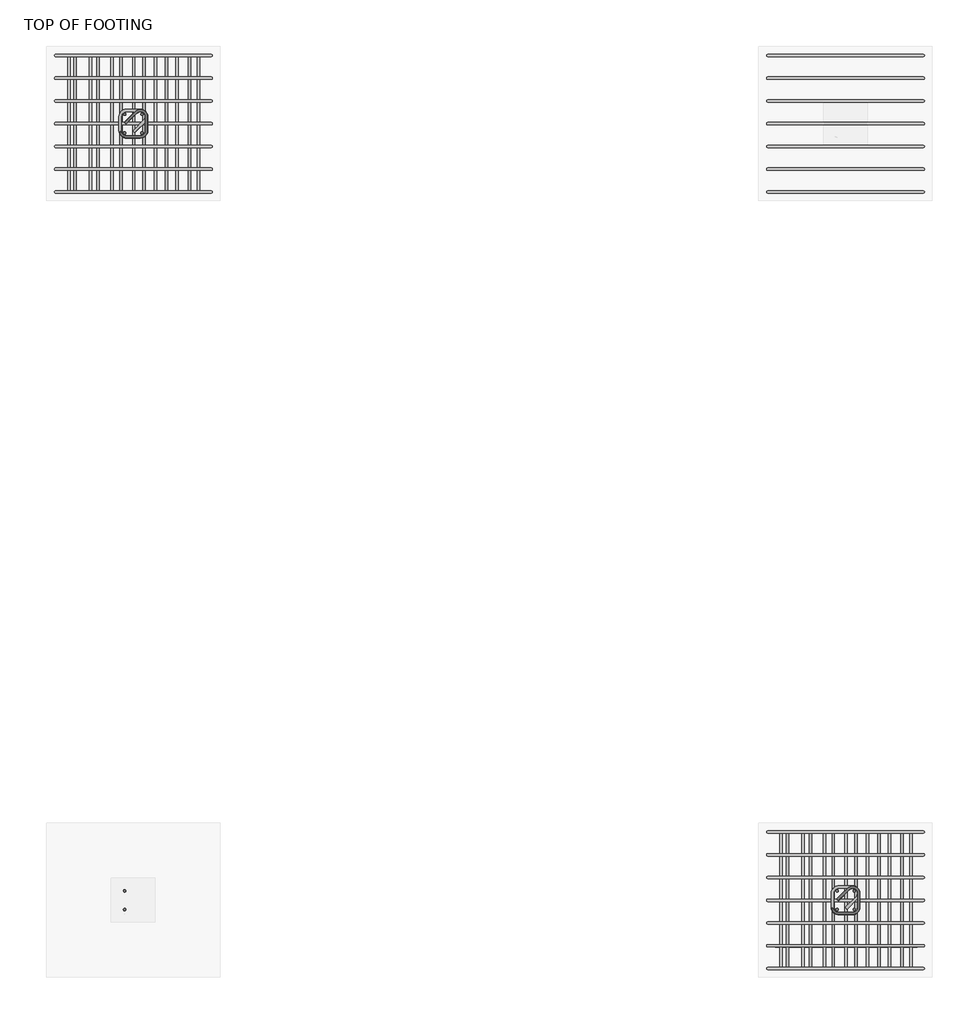
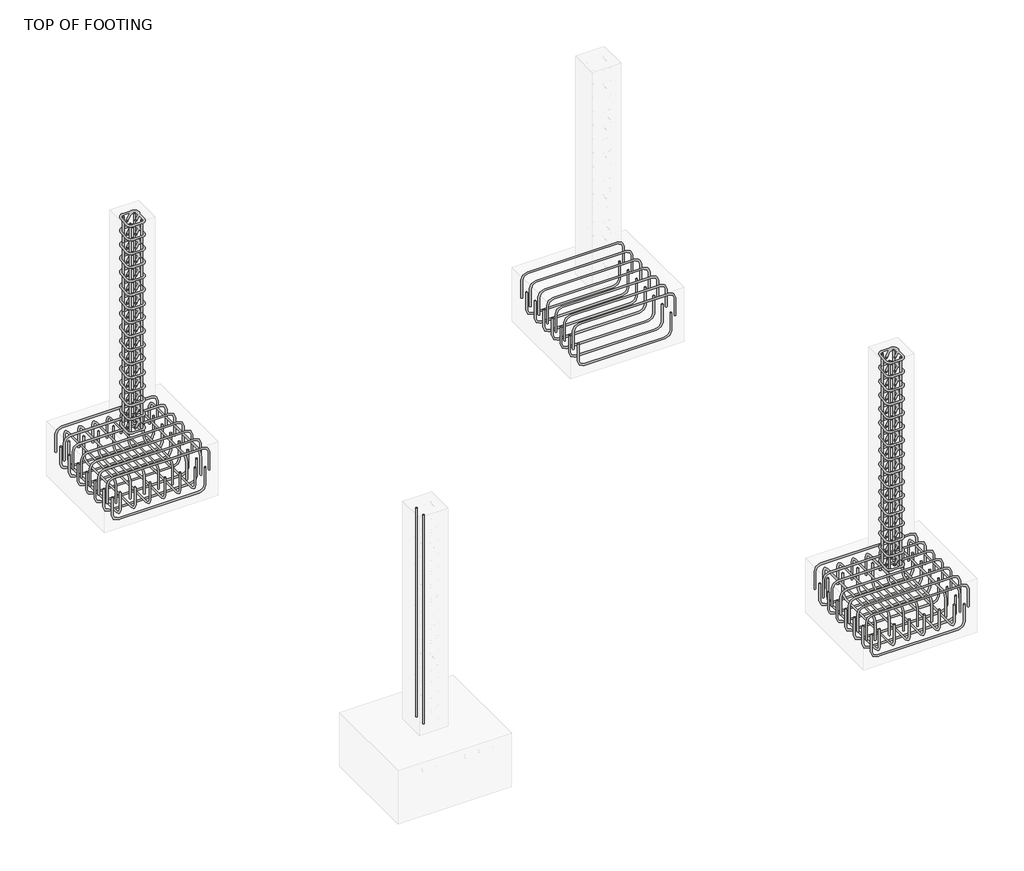
# One storey, part 4 of 6: 17 reinforcing bars.
"""IFC4 building model written with IfcOpenShell, lengths in millimetres."""

from ifc_helpers import new_model, si_unit, point, frame, origin, place, context, project, spatial, polyline, circle_curve, trimmed, segment, composite_curve, source, transform, mapped, element, save
from ifc_brep_helpers import swept_disk

model = new_model("IFC4")

# Units and contexts
model_context = context("Model", 3, world=origin())
ifc_project = project(units=[si_unit("LENGTHUNIT", "METRE", prefix="MILLI")], contexts=[model_context])

# Site, building, storey
site = spatial("IfcSite", under=ifc_project)
building = spatial("IfcBuilding", under=site)
storey = spatial("IfcBuildingStorey", under=building, Name="TOP OF FOOTING", Elevation=-1828.8)

# Reinforcing bars
placement = place(None, origin())
reinforcing_bar_shape = source(origin(), model_context, "Body", "SolidModel", [
    swept_disk(composite_curve([segment(polyline([(-6942.8971795, 120.9474721, -2038.8), (-6942.8971795, 120.9474721, -2186.1)]), True, "CONTINUOUS"), segment(trimmed(circle_curve(frame((-6989.2471795, 120.9474721, -2186.1), z_axis=(0.0, 1.0, 0.0), x_axis=(46.350000000000364, 0.0, 0.0)), 46.35), [point((-6942.8971795, 120.9474721, -2186.1))], [point((-6989.2471795, 120.9474721, -2232.45))], True, "CARTESIAN"), True, "CONTINUOUS"), segment(polyline([(-6989.2471795, 120.9474721, -2232.45), (-7632.3877906, 120.9474721, -2232.45)]), True, "CONTINUOUS"), segment(trimmed(circle_curve(frame((-7632.3877906, 120.9474721, -2186.1), z_axis=(0.0, 1.0, 0.0), x_axis=(0.0, 0.0, -46.34999999999991)), 46.35), [point((-7632.3877906, 120.9474721, -2232.45))], [point((-7678.7377906, 120.9474721, -2186.1))], True, "CARTESIAN"), True, "CONTINUOUS"), segment(polyline([(-7678.7377906, 120.9474721, -2186.1), (-7678.7377906, 120.9474721, -2038.8)]), True, "CONTINUOUS")], self_intersect=False), 6.35),
])
element("IfcReinforcingBar", 1, at=placement, inside=storey, context=model_context, shape_type="MappedRepresentation", body=[
    mapped(reinforcing_bar_shape, transform((0.0, 0.0, 0.0), x_axis=(1.0, 0.0, 0.0), y_axis=(0.0, 1.0, 0.0), z_axis=(0.0, 0.0, 1.0))),
    mapped(reinforcing_bar_shape, transform((0.0, -117.8833333, 0.0), x_axis=(1.0, 0.0, 0.0), y_axis=(0.0, 1.0, 0.0), z_axis=(0.0, 0.0, 1.0))),
    mapped(reinforcing_bar_shape, transform((0.0, -235.7666667, 0.0), x_axis=(1.0, 0.0, 0.0), y_axis=(0.0, 1.0, 0.0), z_axis=(0.0, 0.0, 1.0))),
    mapped(reinforcing_bar_shape, transform((0.0, -353.65, 0.0), x_axis=(1.0, 0.0, 0.0), y_axis=(0.0, 1.0, 0.0), z_axis=(0.0, 0.0, 1.0))),
    mapped(reinforcing_bar_shape, transform((0.0, -471.5333333, 0.0), x_axis=(1.0, 0.0, 0.0), y_axis=(0.0, 1.0, 0.0), z_axis=(0.0, 0.0, 1.0))),
    mapped(reinforcing_bar_shape, transform((0.0, -589.4166667, 0.0), x_axis=(1.0, 0.0, 0.0), y_axis=(0.0, 1.0, 0.0), z_axis=(0.0, 0.0, 1.0))),
    mapped(reinforcing_bar_shape, transform((0.0, -707.3, 0.0), x_axis=(1.0, 0.0, 0.0), y_axis=(0.0, 1.0, 0.0), z_axis=(0.0, 0.0, 1.0))),
])
reinforcing_bar_2_shape = source(origin(), model_context, "Body", "SolidModel", [
    swept_disk(composite_curve([segment(polyline([(-7718.1173382, 120.9474721, -2070.9463075), (-7718.1173382, 120.9474721, -1923.6463075)]), True, "CONTINUOUS"), segment(trimmed(circle_curve(frame((-7671.7673382, 120.9474721, -1923.6463075), z_axis=(0.0, 1.0, 0.0), x_axis=(-46.349999999999454, 0.0, 0.0)), 46.35), [point((-7718.1173382, 120.9474721, -1923.6463075))], [point((-7671.7673382, 120.9474721, -1877.2963075))], True, "CARTESIAN"), True, "CONTINUOUS"), segment(polyline([(-7671.7673382, 120.9474721, -1877.2963075), (-6957.1673382, 120.9474721, -1877.2963075)]), True, "CONTINUOUS"), segment(trimmed(circle_curve(frame((-6957.1673382, 120.9474721, -1923.6463075), z_axis=(0.0, 1.0, 0.0), x_axis=(0.0, 0.0, 46.34999999999991)), 46.35), [point((-6957.1673382, 120.9474721, -1877.2963075))], [point((-6910.8173382, 120.9474721, -1923.6463075))], True, "CARTESIAN"), True, "CONTINUOUS"), segment(polyline([(-6910.8173382, 120.9474721, -1923.6463075), (-6910.8173382, 120.9474721, -2070.9463075)]), True, "CONTINUOUS")], self_intersect=False), 6.35),
])
element("IfcReinforcingBar", 2, at=placement, inside=storey, context=model_context, shape_type="MappedRepresentation", body=[
    mapped(reinforcing_bar_2_shape, transform((0.0, 0.0, 0.0), x_axis=(1.0, 0.0, 0.0), y_axis=(0.0, 1.0, 0.0), z_axis=(0.0, 0.0, 1.0))),
    mapped(reinforcing_bar_2_shape, transform((0.0, -117.8833333, 0.0), x_axis=(1.0, 0.0, 0.0), y_axis=(0.0, 1.0, 0.0), z_axis=(0.0, 0.0, 1.0))),
    mapped(reinforcing_bar_2_shape, transform((0.0, -235.7666667, 0.0), x_axis=(1.0, 0.0, 0.0), y_axis=(0.0, 1.0, 0.0), z_axis=(0.0, 0.0, 1.0))),
    mapped(reinforcing_bar_2_shape, transform((0.0, -353.65, 0.0), x_axis=(1.0, 0.0, 0.0), y_axis=(0.0, 1.0, 0.0), z_axis=(0.0, 0.0, 1.0))),
    mapped(reinforcing_bar_2_shape, transform((0.0, -471.5333333, 0.0), x_axis=(1.0, 0.0, 0.0), y_axis=(0.0, 1.0, 0.0), z_axis=(0.0, 0.0, 1.0))),
    mapped(reinforcing_bar_2_shape, transform((0.0, -589.4166667, 0.0), x_axis=(1.0, 0.0, 0.0), y_axis=(0.0, 1.0, 0.0), z_axis=(0.0, 0.0, 1.0))),
    mapped(reinforcing_bar_2_shape, transform((0.0, -707.3, 0.0), x_axis=(1.0, 0.0, 0.0), y_axis=(0.0, 1.0, 0.0), z_axis=(0.0, 0.0, 1.0))),
])
reinforcing_bar_3_shape = source(origin(), model_context, "Body", "SolidModel", [
    swept_disk(composite_curve([segment(polyline([(-6975.9662545, 120.9474721, -2094.0228735), (-6975.9662545, 120.9474721, -1946.7228735)]), True, "CONTINUOUS"), segment(trimmed(circle_curve(frame((-6975.9662545, 74.5974721, -1946.7228735), z_axis=(1.0, 0.0, 0.0), x_axis=(0.0, 46.349999999999994, 0.0)), 46.35), [point((-6975.9662545, 120.9474721, -1946.7228735))], [point((-6975.9662545, 74.5974721, -1900.3728735))], True, "CARTESIAN"), True, "CONTINUOUS"), segment(polyline([(-6975.9662545, 74.5974721, -1900.3728735), (-6975.9662545, -540.0025279, -1900.3728735)]), True, "CONTINUOUS"), segment(trimmed(circle_curve(frame((-6975.9662545, -540.0025279, -1946.7228735), z_axis=(1.0, 0.0, 0.0), x_axis=(0.0, 0.0, 46.350000000000136)), 46.35), [point((-6975.9662545, -540.0025279, -1900.3728735))], [point((-6975.9662545, -586.3525279, -1946.7228735))], True, "CARTESIAN"), True, "CONTINUOUS"), segment(polyline([(-6975.9662545, -586.3525279, -1946.7228735), (-6975.9662545, -586.3525279, -2094.0228735)]), True, "CONTINUOUS")], self_intersect=False), 6.35),
])
element("IfcReinforcingBar", 3, at=placement, inside=storey, context=model_context, shape_type="MappedRepresentation", body=[
    mapped(reinforcing_bar_3_shape, transform((0.0, 0.0, 0.0), x_axis=(1.0, 0.0, 0.0), y_axis=(0.0, 1.0, 0.0), z_axis=(0.0, 0.0, 1.0))),
    mapped(reinforcing_bar_3_shape, transform((-112.124631, 0.0, 0.0), x_axis=(1.0, 0.0, 0.0), y_axis=(0.0, 1.0, 0.0), z_axis=(0.0, 0.0, 1.0))),
    mapped(reinforcing_bar_3_shape, transform((-224.2492621, 0.0, 0.0), x_axis=(1.0, 0.0, 0.0), y_axis=(0.0, 1.0, 0.0), z_axis=(0.0, 0.0, 1.0))),
    mapped(reinforcing_bar_3_shape, transform((-336.3738931, 0.0, 0.0), x_axis=(1.0, 0.0, 0.0), y_axis=(0.0, 1.0, 0.0), z_axis=(0.0, 0.0, 1.0))),
    mapped(reinforcing_bar_3_shape, transform((-448.4985241, 0.0, 0.0), x_axis=(1.0, 0.0, 0.0), y_axis=(0.0, 1.0, 0.0), z_axis=(0.0, 0.0, 1.0))),
    mapped(reinforcing_bar_3_shape, transform((-560.6231552, 0.0, 0.0), x_axis=(1.0, 0.0, 0.0), y_axis=(0.0, 1.0, 0.0), z_axis=(0.0, 0.0, 1.0))),
    mapped(reinforcing_bar_3_shape, transform((-672.7477862, 0.0, 0.0), x_axis=(1.0, 0.0, 0.0), y_axis=(0.0, 1.0, 0.0), z_axis=(0.0, 0.0, 1.0))),
])
reinforcing_bar_4_shape = source(origin(), model_context, "Body", "SolidModel", [
    swept_disk(composite_curve([segment(polyline([(-7615.9564967, 120.9474721, -2014.7438142), (-7615.9564967, 120.9474721, -2162.0438142)]), True, "CONTINUOUS"), segment(trimmed(circle_curve(frame((-7615.9564967, 74.5974721, -2162.0438142), z_axis=(-1.0, 0.0, 0.0), x_axis=(0.0, 46.349999999999994, 0.0)), 46.35), [point((-7615.9564967, 120.9474721, -2162.0438142))], [point((-7615.9564967, 74.5974721, -2208.3938142))], True, "CARTESIAN"), True, "CONTINUOUS"), segment(polyline([(-7615.9564967, 74.5974721, -2208.3938142), (-7615.9564967, -540.0025279, -2208.3938142)]), True, "CONTINUOUS"), segment(trimmed(circle_curve(frame((-7615.9564967, -540.0025279, -2162.0438142), z_axis=(-1.0, 0.0, 0.0), x_axis=(0.0, 0.0, -46.350000000000364)), 46.35), [point((-7615.9564967, -540.0025279, -2208.3938142))], [point((-7615.9564967, -586.3525279, -2162.0438142))], True, "CARTESIAN"), True, "CONTINUOUS"), segment(polyline([(-7615.9564967, -586.3525279, -2162.0438142), (-7615.9564967, -586.3525279, -2014.7438142)]), True, "CONTINUOUS")], self_intersect=False), 6.35),
])
element("IfcReinforcingBar", 4, at=placement, inside=storey, context=model_context, shape_type="MappedRepresentation", body=[
    mapped(reinforcing_bar_4_shape, transform((0.0, 0.0, 0.0), x_axis=(1.0, 0.0, 0.0), y_axis=(0.0, 1.0, 0.0), z_axis=(0.0, 0.0, 1.0))),
    mapped(reinforcing_bar_4_shape, transform((118.647936, 0.0, 0.0), x_axis=(1.0, 0.0, 0.0), y_axis=(0.0, 1.0, 0.0), z_axis=(0.0, 0.0, 1.0))),
    mapped(reinforcing_bar_4_shape, transform((237.295872, 0.0, 0.0), x_axis=(1.0, 0.0, 0.0), y_axis=(0.0, 1.0, 0.0), z_axis=(0.0, 0.0, 1.0))),
    mapped(reinforcing_bar_4_shape, transform((355.943808, 0.0, 0.0), x_axis=(1.0, 0.0, 0.0), y_axis=(0.0, 1.0, 0.0), z_axis=(0.0, 0.0, 1.0))),
    mapped(reinforcing_bar_4_shape, transform((474.591744, 0.0, 0.0), x_axis=(1.0, 0.0, 0.0), y_axis=(0.0, 1.0, 0.0), z_axis=(0.0, 0.0, 1.0))),
    mapped(reinforcing_bar_4_shape, transform((593.23968, 0.0, 0.0), x_axis=(1.0, 0.0, 0.0), y_axis=(0.0, 1.0, 0.0), z_axis=(0.0, 0.0, 1.0))),
])
reinforcing_bar_5_shape = source(origin(), model_context, "Body", "SolidModel", [
    swept_disk(composite_curve([segment(polyline([(-3249.1855212, -3906.2483349, -2038.8), (-3249.1855212, -3906.2483349, -2186.1)]), True, "CONTINUOUS"), segment(trimmed(circle_curve(frame((-3295.5355212, -3906.2483349, -2186.1), z_axis=(0.0, 1.0, 0.0), x_axis=(46.34999999999991, 0.0, 0.0)), 46.35), [point((-3249.1855212, -3906.2483349, -2186.1))], [point((-3295.5355212, -3906.2483349, -2232.45))], True, "CARTESIAN"), True, "CONTINUOUS"), segment(polyline([(-3295.5355212, -3906.2483349, -2232.45), (-3938.6761323, -3906.2483349, -2232.45)]), True, "CONTINUOUS"), segment(trimmed(circle_curve(frame((-3938.6761323, -3906.2483349, -2186.1), z_axis=(0.0, 1.0, 0.0), x_axis=(0.0, 0.0, -46.34999999999991)), 46.35), [point((-3938.6761323, -3906.2483349, -2232.45))], [point((-3985.0261323, -3906.2483349, -2186.1))], True, "CARTESIAN"), True, "CONTINUOUS"), segment(polyline([(-3985.0261323, -3906.2483349, -2186.1), (-3985.0261323, -3906.2483349, -2038.8)]), True, "CONTINUOUS")], self_intersect=False), 6.35),
])
element("IfcReinforcingBar", 5, at=placement, inside=storey, context=model_context, shape_type="MappedRepresentation", body=[
    mapped(reinforcing_bar_5_shape, transform((0.0, 0.0, 0.0), x_axis=(1.0, 0.0, 0.0), y_axis=(0.0, 1.0, 0.0), z_axis=(0.0, 0.0, 1.0))),
    mapped(reinforcing_bar_5_shape, transform((0.0, -117.8833333, 0.0), x_axis=(1.0, 0.0, 0.0), y_axis=(0.0, 1.0, 0.0), z_axis=(0.0, 0.0, 1.0))),
    mapped(reinforcing_bar_5_shape, transform((0.0, -235.7666667, 0.0), x_axis=(1.0, 0.0, 0.0), y_axis=(0.0, 1.0, 0.0), z_axis=(0.0, 0.0, 1.0))),
    mapped(reinforcing_bar_5_shape, transform((0.0, -353.65, 0.0), x_axis=(1.0, 0.0, 0.0), y_axis=(0.0, 1.0, 0.0), z_axis=(0.0, 0.0, 1.0))),
    mapped(reinforcing_bar_5_shape, transform((0.0, -471.5333333, 0.0), x_axis=(1.0, 0.0, 0.0), y_axis=(0.0, 1.0, 0.0), z_axis=(0.0, 0.0, 1.0))),
    mapped(reinforcing_bar_5_shape, transform((0.0, -589.4166667, 0.0), x_axis=(1.0, 0.0, 0.0), y_axis=(0.0, 1.0, 0.0), z_axis=(0.0, 0.0, 1.0))),
    mapped(reinforcing_bar_5_shape, transform((0.0, -707.3, 0.0), x_axis=(1.0, 0.0, 0.0), y_axis=(0.0, 1.0, 0.0), z_axis=(0.0, 0.0, 1.0))),
])
reinforcing_bar_6_shape = source(origin(), model_context, "Body", "SolidModel", [
    swept_disk(composite_curve([segment(polyline([(-4024.4056799, -3906.2483349, -2070.9463075), (-4024.4056799, -3906.2483349, -1923.6463075)]), True, "CONTINUOUS"), segment(trimmed(circle_curve(frame((-3978.0556799, -3906.2483349, -1923.6463075), z_axis=(0.0, 1.0, 0.0), x_axis=(-46.34999999999991, 0.0, 0.0)), 46.35), [point((-4024.4056799, -3906.2483349, -1923.6463075))], [point((-3978.0556799, -3906.2483349, -1877.2963075))], True, "CARTESIAN"), True, "CONTINUOUS"), segment(polyline([(-3978.0556799, -3906.2483349, -1877.2963075), (-3263.4556799, -3906.2483349, -1877.2963075)]), True, "CONTINUOUS"), segment(trimmed(circle_curve(frame((-3263.4556799, -3906.2483349, -1923.6463075), z_axis=(0.0, 1.0, 0.0), x_axis=(0.0, 0.0, 46.34999999999991)), 46.35), [point((-3263.4556799, -3906.2483349, -1877.2963075))], [point((-3217.1056799, -3906.2483349, -1923.6463075))], True, "CARTESIAN"), True, "CONTINUOUS"), segment(polyline([(-3217.1056799, -3906.2483349, -1923.6463075), (-3217.1056799, -3906.2483349, -2070.9463075)]), True, "CONTINUOUS")], self_intersect=False), 6.35),
])
element("IfcReinforcingBar", 6, at=placement, inside=storey, context=model_context, shape_type="MappedRepresentation", body=[
    mapped(reinforcing_bar_6_shape, transform((0.0, 0.0, 0.0), x_axis=(1.0, 0.0, 0.0), y_axis=(0.0, 1.0, 0.0), z_axis=(0.0, 0.0, 1.0))),
    mapped(reinforcing_bar_6_shape, transform((0.0, -117.8833333, 0.0), x_axis=(1.0, 0.0, 0.0), y_axis=(0.0, 1.0, 0.0), z_axis=(0.0, 0.0, 1.0))),
    mapped(reinforcing_bar_6_shape, transform((0.0, -235.7666667, 0.0), x_axis=(1.0, 0.0, 0.0), y_axis=(0.0, 1.0, 0.0), z_axis=(0.0, 0.0, 1.0))),
    mapped(reinforcing_bar_6_shape, transform((0.0, -353.65, 0.0), x_axis=(1.0, 0.0, 0.0), y_axis=(0.0, 1.0, 0.0), z_axis=(0.0, 0.0, 1.0))),
    mapped(reinforcing_bar_6_shape, transform((0.0, -471.5333333, 0.0), x_axis=(1.0, 0.0, 0.0), y_axis=(0.0, 1.0, 0.0), z_axis=(0.0, 0.0, 1.0))),
    mapped(reinforcing_bar_6_shape, transform((0.0, -589.4166667, 0.0), x_axis=(1.0, 0.0, 0.0), y_axis=(0.0, 1.0, 0.0), z_axis=(0.0, 0.0, 1.0))),
    mapped(reinforcing_bar_6_shape, transform((0.0, -707.3, 0.0), x_axis=(1.0, 0.0, 0.0), y_axis=(0.0, 1.0, 0.0), z_axis=(0.0, 0.0, 1.0))),
])
reinforcing_bar_7_shape = source(origin(), model_context, "Body", "SolidModel", [
    swept_disk(composite_curve([segment(polyline([(-3282.2545962, -3906.2483349, -2094.0228735), (-3282.2545962, -3906.2483349, -1946.7228735)]), True, "CONTINUOUS"), segment(trimmed(circle_curve(frame((-3282.2545962, -3952.5983349, -1946.7228735), z_axis=(1.0, 0.0, 0.0), x_axis=(0.0, 46.34999999999991, 0.0)), 46.35), [point((-3282.2545962, -3906.2483349, -1946.7228735))], [point((-3282.2545962, -3952.5983349, -1900.3728735))], True, "CARTESIAN"), True, "CONTINUOUS"), segment(polyline([(-3282.2545962, -3952.5983349, -1900.3728735), (-3282.2545962, -4567.1983349, -1900.3728735)]), True, "CONTINUOUS"), segment(trimmed(circle_curve(frame((-3282.2545962, -4567.1983349, -1946.7228735), z_axis=(1.0, 0.0, 0.0), x_axis=(0.0, 0.0, 46.350000000000136)), 46.35), [point((-3282.2545962, -4567.1983349, -1900.3728735))], [point((-3282.2545962, -4613.5483349, -1946.7228735))], True, "CARTESIAN"), True, "CONTINUOUS"), segment(polyline([(-3282.2545962, -4613.5483349, -1946.7228735), (-3282.2545962, -4613.5483349, -2094.0228735)]), True, "CONTINUOUS")], self_intersect=False), 6.35),
])
element("IfcReinforcingBar", 7, at=placement, inside=storey, context=model_context, shape_type="MappedRepresentation", body=[
    mapped(reinforcing_bar_7_shape, transform((0.0, 0.0, 0.0), x_axis=(1.0, 0.0, 0.0), y_axis=(0.0, 1.0, 0.0), z_axis=(0.0, 0.0, 1.0))),
    mapped(reinforcing_bar_7_shape, transform((-112.124631, 0.0, 0.0), x_axis=(1.0, 0.0, 0.0), y_axis=(0.0, 1.0, 0.0), z_axis=(0.0, 0.0, 1.0))),
    mapped(reinforcing_bar_7_shape, transform((-224.2492621, 0.0, 0.0), x_axis=(1.0, 0.0, 0.0), y_axis=(0.0, 1.0, 0.0), z_axis=(0.0, 0.0, 1.0))),
    mapped(reinforcing_bar_7_shape, transform((-336.3738931, 0.0, 0.0), x_axis=(1.0, 0.0, 0.0), y_axis=(0.0, 1.0, 0.0), z_axis=(0.0, 0.0, 1.0))),
    mapped(reinforcing_bar_7_shape, transform((-448.4985241, 0.0, 0.0), x_axis=(1.0, 0.0, 0.0), y_axis=(0.0, 1.0, 0.0), z_axis=(0.0, 0.0, 1.0))),
    mapped(reinforcing_bar_7_shape, transform((-560.6231552, 0.0, 0.0), x_axis=(1.0, 0.0, 0.0), y_axis=(0.0, 1.0, 0.0), z_axis=(0.0, 0.0, 1.0))),
    mapped(reinforcing_bar_7_shape, transform((-672.7477862, 0.0, 0.0), x_axis=(1.0, 0.0, 0.0), y_axis=(0.0, 1.0, 0.0), z_axis=(0.0, 0.0, 1.0))),
])
reinforcing_bar_8_shape = source(origin(), model_context, "Body", "SolidModel", [
    swept_disk(composite_curve([segment(polyline([(-3922.2448384, -3906.2483349, -2014.7438142), (-3922.2448384, -3906.2483349, -2162.0438142)]), True, "CONTINUOUS"), segment(trimmed(circle_curve(frame((-3922.2448384, -3952.5983349, -2162.0438142), z_axis=(-1.0, 0.0, 0.0), x_axis=(0.0, 46.34999999999991, 0.0)), 46.35), [point((-3922.2448384, -3906.2483349, -2162.0438142))], [point((-3922.2448384, -3952.5983349, -2208.3938142))], True, "CARTESIAN"), True, "CONTINUOUS"), segment(polyline([(-3922.2448384, -3952.5983349, -2208.3938142), (-3922.2448384, -4567.1983349, -2208.3938142)]), True, "CONTINUOUS"), segment(trimmed(circle_curve(frame((-3922.2448384, -4567.1983349, -2162.0438142), z_axis=(-1.0, 0.0, 0.0), x_axis=(0.0, 0.0, -46.350000000000364)), 46.35), [point((-3922.2448384, -4567.1983349, -2208.3938142))], [point((-3922.2448384, -4613.5483349, -2162.0438142))], True, "CARTESIAN"), True, "CONTINUOUS"), segment(polyline([(-3922.2448384, -4613.5483349, -2162.0438142), (-3922.2448384, -4613.5483349, -2014.7438142)]), True, "CONTINUOUS")], self_intersect=False), 6.35),
])
element("IfcReinforcingBar", 8, at=placement, inside=storey, context=model_context, shape_type="MappedRepresentation", body=[
    mapped(reinforcing_bar_8_shape, transform((0.0, 0.0, 0.0), x_axis=(1.0, 0.0, 0.0), y_axis=(0.0, 1.0, 0.0), z_axis=(0.0, 0.0, 1.0))),
    mapped(reinforcing_bar_8_shape, transform((118.647936, 0.0, 0.0), x_axis=(1.0, 0.0, 0.0), y_axis=(0.0, 1.0, 0.0), z_axis=(0.0, 0.0, 1.0))),
    mapped(reinforcing_bar_8_shape, transform((237.295872, 0.0, 0.0), x_axis=(1.0, 0.0, 0.0), y_axis=(0.0, 1.0, 0.0), z_axis=(0.0, 0.0, 1.0))),
    mapped(reinforcing_bar_8_shape, transform((355.943808, 0.0, 0.0), x_axis=(1.0, 0.0, 0.0), y_axis=(0.0, 1.0, 0.0), z_axis=(0.0, 0.0, 1.0))),
    mapped(reinforcing_bar_8_shape, transform((474.591744, 0.0, 0.0), x_axis=(1.0, 0.0, 0.0), y_axis=(0.0, 1.0, 0.0), z_axis=(0.0, 0.0, 1.0))),
    mapped(reinforcing_bar_8_shape, transform((593.23968, 0.0, 0.0), x_axis=(1.0, 0.0, 0.0), y_axis=(0.0, 1.0, 0.0), z_axis=(0.0, 0.0, 1.0))),
])
reinforcing_bar_9_shape = source(origin(), model_context, "Body", "SolidModel", [
    swept_disk(composite_curve([segment(polyline([(-3249.1855212, 120.9474721, -2038.8), (-3249.1855212, 120.9474721, -2186.1)]), True, "CONTINUOUS"), segment(trimmed(circle_curve(frame((-3295.5355212, 120.9474721, -2186.1), z_axis=(0.0, 1.0, 0.0), x_axis=(46.34999999999991, 0.0, 0.0)), 46.35), [point((-3249.1855212, 120.9474721, -2186.1))], [point((-3295.5355212, 120.9474721, -2232.45))], True, "CARTESIAN"), True, "CONTINUOUS"), segment(polyline([(-3295.5355212, 120.9474721, -2232.45), (-3938.6761323, 120.9474721, -2232.45)]), True, "CONTINUOUS"), segment(trimmed(circle_curve(frame((-3938.6761323, 120.9474721, -2186.1), z_axis=(0.0, 1.0, 0.0), x_axis=(0.0, 0.0, -46.34999999999991)), 46.35), [point((-3938.6761323, 120.9474721, -2232.45))], [point((-3985.0261323, 120.9474721, -2186.1))], True, "CARTESIAN"), True, "CONTINUOUS"), segment(polyline([(-3985.0261323, 120.9474721, -2186.1), (-3985.0261323, 120.9474721, -2038.8)]), True, "CONTINUOUS")], self_intersect=False), 6.35),
])
element("IfcReinforcingBar", 9, at=placement, inside=storey, context=model_context, shape_type="MappedRepresentation", body=[
    mapped(reinforcing_bar_9_shape, transform((0.0, 0.0, 0.0), x_axis=(1.0, 0.0, 0.0), y_axis=(0.0, 1.0, 0.0), z_axis=(0.0, 0.0, 1.0))),
    mapped(reinforcing_bar_9_shape, transform((0.0, -117.8833333, 0.0), x_axis=(1.0, 0.0, 0.0), y_axis=(0.0, 1.0, 0.0), z_axis=(0.0, 0.0, 1.0))),
    mapped(reinforcing_bar_9_shape, transform((0.0, -235.7666667, 0.0), x_axis=(1.0, 0.0, 0.0), y_axis=(0.0, 1.0, 0.0), z_axis=(0.0, 0.0, 1.0))),
    mapped(reinforcing_bar_9_shape, transform((0.0, -353.65, 0.0), x_axis=(1.0, 0.0, 0.0), y_axis=(0.0, 1.0, 0.0), z_axis=(0.0, 0.0, 1.0))),
    mapped(reinforcing_bar_9_shape, transform((0.0, -471.5333333, 0.0), x_axis=(1.0, 0.0, 0.0), y_axis=(0.0, 1.0, 0.0), z_axis=(0.0, 0.0, 1.0))),
    mapped(reinforcing_bar_9_shape, transform((0.0, -589.4166667, 0.0), x_axis=(1.0, 0.0, 0.0), y_axis=(0.0, 1.0, 0.0), z_axis=(0.0, 0.0, 1.0))),
    mapped(reinforcing_bar_9_shape, transform((0.0, -707.3, 0.0), x_axis=(1.0, 0.0, 0.0), y_axis=(0.0, 1.0, 0.0), z_axis=(0.0, 0.0, 1.0))),
])
reinforcing_bar_10_shape = source(origin(), model_context, "Body", "SolidModel", [
    swept_disk(composite_curve([segment(polyline([(-4024.4056799, 120.9474721, -2070.9463075), (-4024.4056799, 120.9474721, -1923.6463075)]), True, "CONTINUOUS"), segment(trimmed(circle_curve(frame((-3978.0556799, 120.9474721, -1923.6463075), z_axis=(0.0, 1.0, 0.0), x_axis=(-46.34999999999991, 0.0, 0.0)), 46.35), [point((-4024.4056799, 120.9474721, -1923.6463075))], [point((-3978.0556799, 120.9474721, -1877.2963075))], True, "CARTESIAN"), True, "CONTINUOUS"), segment(polyline([(-3978.0556799, 120.9474721, -1877.2963075), (-3263.4556799, 120.9474721, -1877.2963075)]), True, "CONTINUOUS"), segment(trimmed(circle_curve(frame((-3263.4556799, 120.9474721, -1923.6463075), z_axis=(0.0, 1.0, 0.0), x_axis=(0.0, 0.0, 46.34999999999991)), 46.35), [point((-3263.4556799, 120.9474721, -1877.2963075))], [point((-3217.1056799, 120.9474721, -1923.6463075))], True, "CARTESIAN"), True, "CONTINUOUS"), segment(polyline([(-3217.1056799, 120.9474721, -1923.6463075), (-3217.1056799, 120.9474721, -2070.9463075)]), True, "CONTINUOUS")], self_intersect=False), 6.35),
])
element("IfcReinforcingBar", 10, at=placement, inside=storey, context=model_context, shape_type="MappedRepresentation", body=[
    mapped(reinforcing_bar_10_shape, transform((0.0, 0.0, 0.0), x_axis=(1.0, 0.0, 0.0), y_axis=(0.0, 1.0, 0.0), z_axis=(0.0, 0.0, 1.0))),
    mapped(reinforcing_bar_10_shape, transform((0.0, -117.8833333, 0.0), x_axis=(1.0, 0.0, 0.0), y_axis=(0.0, 1.0, 0.0), z_axis=(0.0, 0.0, 1.0))),
    mapped(reinforcing_bar_10_shape, transform((0.0, -235.7666667, 0.0), x_axis=(1.0, 0.0, 0.0), y_axis=(0.0, 1.0, 0.0), z_axis=(0.0, 0.0, 1.0))),
    mapped(reinforcing_bar_10_shape, transform((0.0, -353.65, 0.0), x_axis=(1.0, 0.0, 0.0), y_axis=(0.0, 1.0, 0.0), z_axis=(0.0, 0.0, 1.0))),
    mapped(reinforcing_bar_10_shape, transform((0.0, -471.5333333, 0.0), x_axis=(1.0, 0.0, 0.0), y_axis=(0.0, 1.0, 0.0), z_axis=(0.0, 0.0, 1.0))),
    mapped(reinforcing_bar_10_shape, transform((0.0, -589.4166667, 0.0), x_axis=(1.0, 0.0, 0.0), y_axis=(0.0, 1.0, 0.0), z_axis=(0.0, 0.0, 1.0))),
    mapped(reinforcing_bar_10_shape, transform((0.0, -707.3, 0.0), x_axis=(1.0, 0.0, 0.0), y_axis=(0.0, 1.0, 0.0), z_axis=(0.0, 0.0, 1.0))),
])
reinforcing_bar_11_shape = source(origin(), model_context, "Body", "SolidModel", [
    swept_disk(composite_curve([segment(polyline([(-7359.2223245, -4211.1006392, -40.0), (-7359.2223245, -4211.1006392, -1788.8)]), True, "CONTINUOUS")], self_intersect=False), 6.35),
])
element("IfcReinforcingBar", 11, at=placement, inside=storey, context=model_context, shape_type="MappedRepresentation", body=[
    mapped(reinforcing_bar_11_shape, transform((0.0, 0.0, 0.0), x_axis=(1.0, 0.0, 0.0), y_axis=(0.0, 1.0, 0.0), z_axis=(0.0, 0.0, 1.0))),
    mapped(reinforcing_bar_11_shape, transform((0.0, -96.9916148, 0.0), x_axis=(1.0, 0.0, 0.0), y_axis=(0.0, 1.0, 0.0), z_axis=(0.0, 0.0, 1.0))),
])
reinforcing_bar_12_shape = source(origin(), model_context, "Body", "SolidModel", [
    swept_disk(composite_curve([segment(polyline([(-3576.0006936, -4211.1006392, -40.0), (-3576.0006936, -4211.1006392, -1788.8)]), True, "CONTINUOUS")], self_intersect=False), 6.35),
])
element("IfcReinforcingBar", 12, at=placement, inside=storey, context=model_context, shape_type="MappedRepresentation", body=[
    mapped(reinforcing_bar_12_shape, transform((0.0, 0.0, 0.0), x_axis=(1.0, 0.0, 0.0), y_axis=(0.0, 1.0, 0.0), z_axis=(0.0, 0.0, 1.0))),
    mapped(reinforcing_bar_12_shape, transform((0.0, -96.9916148, 0.0), x_axis=(1.0, 0.0, 0.0), y_axis=(0.0, 1.0, 0.0), z_axis=(0.0, 0.0, 1.0))),
])
reinforcing_bar_13_shape = source(origin(), model_context, "Body", "SolidModel", [
    swept_disk(composite_curve([segment(polyline([(-3662.0670404, -4256.8741003, -46.35), (-3606.3234775, -4201.1305373, -46.35)]), True, "CONTINUOUS"), segment(trimmed(circle_curve(frame((-3584.1556799, -4223.2983349, -46.35), z_axis=(0.0, 0.0, -1.0), x_axis=(-22.167797600000085, 22.167797600000085, 0.0)), 31.35), [point((-3606.3234775, -4201.1305373, -46.35))], [point((-3552.8056799, -4223.2983349, -46.35))], True, "CARTESIAN"), True, "CONTINUOUS"), segment(polyline([(-3552.8056799, -4223.2983349, -46.35), (-3552.8056799, -4296.4983349, -46.35)]), True, "CONTINUOUS"), segment(trimmed(circle_curve(frame((-3584.1556799, -4296.4983349, -46.35), z_axis=(0.0, 0.0, -1.0), x_axis=(31.34999999999991, 0.0, 0.0)), 31.35), [point((-3552.8056799, -4296.4983349, -46.35))], [point((-3584.1556799, -4327.8483349, -46.35))], True, "CARTESIAN"), True, "CONTINUOUS"), segment(polyline([(-3584.1556799, -4327.8483349, -46.35), (-3657.3556799, -4327.8483349, -46.35)]), True, "CONTINUOUS"), segment(trimmed(circle_curve(frame((-3657.3556799, -4296.6343361, -43.4330185), z_axis=(0.0, 0.09304566152621355, -0.9956618426308951), x_axis=(0.0, -31.2139987999999, -2.9169814999999986)), 31.35), [point((-3657.3556799, -4327.8483349, -46.35))], [point((-3688.7056799, -4296.6343361, -43.4330185))], True, "CARTESIAN"), True, "CONTINUOUS"), segment(polyline([(-3688.7056799, -4296.6343361, -43.4330185), (-3688.7056799, -4223.1623337, -36.5669815)]), True, "CONTINUOUS"), segment(trimmed(circle_curve(frame((-3657.3556799, -4223.1623337, -36.5669815), z_axis=(0.0, 0.09304566152621355, -0.9956618426308951), x_axis=(-31.350000000000364, 0.0, 0.0)), 31.35), [point((-3688.7056799, -4223.1623337, -36.5669815))], [point((-3657.3556799, -4191.9483349, -33.65))], True, "CARTESIAN"), True, "CONTINUOUS"), segment(polyline([(-3657.3556799, -4191.9483349, -33.65), (-3584.1556799, -4191.9483349, -33.65)]), True, "CONTINUOUS"), segment(trimmed(circle_curve(frame((-3584.1556799, -4223.2983349, -33.65), z_axis=(0.0, 0.0, -1.0), x_axis=(0.0, 31.349999999999454, 0.0)), 31.35), [point((-3584.1556799, -4191.9483349, -33.65))], [point((-3561.9878823, -4245.4661325, -33.65))], True, "CARTESIAN"), True, "CONTINUOUS"), segment(polyline([(-3561.9878823, -4245.4661325, -33.65), (-3617.7314452, -4301.2096954, -33.65)]), True, "CONTINUOUS")], self_intersect=False), 6.35),
])
element("IfcReinforcingBar", 13, at=placement, inside=storey, context=model_context, shape_type="MappedRepresentation", body=[
    mapped(reinforcing_bar_13_shape, transform((0.0, 0.0, 0.0), x_axis=(1.0, 0.0, 0.0), y_axis=(0.0, 1.0, 0.0), z_axis=(0.0, 0.0, 1.0))),
    mapped(reinforcing_bar_13_shape, transform((0.0, 0.0, -115.74), x_axis=(1.0, 0.0, 0.0), y_axis=(0.0, 1.0, 0.0), z_axis=(0.0, 0.0, 1.0))),
    mapped(reinforcing_bar_13_shape, transform((0.0, 0.0, -231.48), x_axis=(1.0, 0.0, 0.0), y_axis=(0.0, 1.0, 0.0), z_axis=(0.0, 0.0, 1.0))),
    mapped(reinforcing_bar_13_shape, transform((0.0, 0.0, -347.22), x_axis=(1.0, 0.0, 0.0), y_axis=(0.0, 1.0, 0.0), z_axis=(0.0, 0.0, 1.0))),
    mapped(reinforcing_bar_13_shape, transform((0.0, 0.0, -462.96), x_axis=(1.0, 0.0, 0.0), y_axis=(0.0, 1.0, 0.0), z_axis=(0.0, 0.0, 1.0))),
    mapped(reinforcing_bar_13_shape, transform((0.0, 0.0, -578.7), x_axis=(1.0, 0.0, 0.0), y_axis=(0.0, 1.0, 0.0), z_axis=(0.0, 0.0, 1.0))),
    mapped(reinforcing_bar_13_shape, transform((0.0, 0.0, -694.44), x_axis=(1.0, 0.0, 0.0), y_axis=(0.0, 1.0, 0.0), z_axis=(0.0, 0.0, 1.0))),
    mapped(reinforcing_bar_13_shape, transform((0.0, 0.0, -810.18), x_axis=(1.0, 0.0, 0.0), y_axis=(0.0, 1.0, 0.0), z_axis=(0.0, 0.0, 1.0))),
    mapped(reinforcing_bar_13_shape, transform((0.0, 0.0, -925.92), x_axis=(1.0, 0.0, 0.0), y_axis=(0.0, 1.0, 0.0), z_axis=(0.0, 0.0, 1.0))),
    mapped(reinforcing_bar_13_shape, transform((0.0, 0.0, -1041.66), x_axis=(1.0, 0.0, 0.0), y_axis=(0.0, 1.0, 0.0), z_axis=(0.0, 0.0, 1.0))),
    mapped(reinforcing_bar_13_shape, transform((0.0, 0.0, -1157.4), x_axis=(1.0, 0.0, 0.0), y_axis=(0.0, 1.0, 0.0), z_axis=(0.0, 0.0, 1.0))),
    mapped(reinforcing_bar_13_shape, transform((0.0, 0.0, -1273.14), x_axis=(1.0, 0.0, 0.0), y_axis=(0.0, 1.0, 0.0), z_axis=(0.0, 0.0, 1.0))),
    mapped(reinforcing_bar_13_shape, transform((0.0, 0.0, -1388.88), x_axis=(1.0, 0.0, 0.0), y_axis=(0.0, 1.0, 0.0), z_axis=(0.0, 0.0, 1.0))),
    mapped(reinforcing_bar_13_shape, transform((0.0, 0.0, -1504.62), x_axis=(1.0, 0.0, 0.0), y_axis=(0.0, 1.0, 0.0), z_axis=(0.0, 0.0, 1.0))),
    mapped(reinforcing_bar_13_shape, transform((0.0, 0.0, -1620.36), x_axis=(1.0, 0.0, 0.0), y_axis=(0.0, 1.0, 0.0), z_axis=(0.0, 0.0, 1.0))),
    mapped(reinforcing_bar_13_shape, transform((0.0, 0.0, -1736.1), x_axis=(1.0, 0.0, 0.0), y_axis=(0.0, 1.0, 0.0), z_axis=(0.0, 0.0, 1.0))),
])
reinforcing_bar_14_shape = source(origin(), model_context, "Body", "SolidModel", [
    swept_disk(composite_curve([segment(polyline([(-3665.5106662, -4211.1006392, -40.0), (-3665.5106662, -4211.1006392, -1788.8)]), True, "CONTINUOUS")], self_intersect=False), 6.35),
])
element("IfcReinforcingBar", 14, at=placement, inside=storey, context=model_context, shape_type="MappedRepresentation", body=[
    mapped(reinforcing_bar_14_shape, transform((0.0, 0.0, 0.0), x_axis=(1.0, 0.0, 0.0), y_axis=(0.0, 1.0, 0.0), z_axis=(0.0, 0.0, 1.0))),
    mapped(reinforcing_bar_14_shape, transform((0.0, -96.9916148, 0.0), x_axis=(1.0, 0.0, 0.0), y_axis=(0.0, 1.0, 0.0), z_axis=(0.0, 0.0, 1.0))),
])
reinforcing_bar_15_shape = source(origin(), model_context, "Body", "SolidModel", [
    swept_disk(composite_curve([segment(polyline([(-7269.7123519, -183.9048321, -40.0), (-7269.7123519, -183.9048321, -1788.8)]), True, "CONTINUOUS")], self_intersect=False), 6.35),
])
element("IfcReinforcingBar", 15, at=placement, inside=storey, context=model_context, shape_type="MappedRepresentation", body=[
    mapped(reinforcing_bar_15_shape, transform((0.0, 0.0, 0.0), x_axis=(1.0, 0.0, 0.0), y_axis=(0.0, 1.0, 0.0), z_axis=(0.0, 0.0, 1.0))),
    mapped(reinforcing_bar_15_shape, transform((0.0, -96.9916148, 0.0), x_axis=(1.0, 0.0, 0.0), y_axis=(0.0, 1.0, 0.0), z_axis=(0.0, 0.0, 1.0))),
])
reinforcing_bar_16_shape = source(origin(), model_context, "Body", "SolidModel", [
    swept_disk(composite_curve([segment(polyline([(-7355.7786987, -229.6782932, -46.35), (-7300.0351358, -173.9347303, -46.35)]), True, "CONTINUOUS"), segment(trimmed(circle_curve(frame((-7277.8673382, -196.1025279, -46.35), z_axis=(0.0, 0.0, -1.0), x_axis=(-22.167797600000085, 22.1677976, 0.0)), 31.35), [point((-7300.0351358, -173.9347303, -46.35))], [point((-7246.5173382, -196.1025279, -46.35))], True, "CARTESIAN"), True, "CONTINUOUS"), segment(polyline([(-7246.5173382, -196.1025279, -46.35), (-7246.5173382, -269.3025279, -46.35)]), True, "CONTINUOUS"), segment(trimmed(circle_curve(frame((-7277.8673382, -269.3025279, -46.35), z_axis=(0.0, 0.0, -1.0), x_axis=(31.349999999999454, 0.0, 0.0)), 31.35), [point((-7246.5173382, -269.3025279, -46.35))], [point((-7277.8673382, -300.6525279, -46.35))], True, "CARTESIAN"), True, "CONTINUOUS"), segment(polyline([(-7277.8673382, -300.6525279, -46.35), (-7351.0673382, -300.6525279, -46.35)]), True, "CONTINUOUS"), segment(trimmed(circle_curve(frame((-7351.0673382, -269.4385291, -43.4330185), z_axis=(0.0, 0.09304566152621355, -0.9956618426308951), x_axis=(0.0, -31.213998800000013, -2.9169814999999986)), 31.35), [point((-7351.0673382, -300.6525279, -46.35))], [point((-7382.4173382, -269.4385291, -43.4330185))], True, "CARTESIAN"), True, "CONTINUOUS"), segment(polyline([(-7382.4173382, -269.4385291, -43.4330185), (-7382.4173382, -195.9665266, -36.5669815)]), True, "CONTINUOUS"), segment(trimmed(circle_curve(frame((-7351.0673382, -195.9665266, -36.5669815), z_axis=(0.0, 0.09304566152621355, -0.9956618426308951), x_axis=(-31.349999999999454, 0.0, 0.0)), 31.35), [point((-7382.4173382, -195.9665266, -36.5669815))], [point((-7351.0673382, -164.7525279, -33.65))], True, "CARTESIAN"), True, "CONTINUOUS"), segment(polyline([(-7351.0673382, -164.7525279, -33.65), (-7277.8673382, -164.7525279, -33.65)]), True, "CONTINUOUS"), segment(trimmed(circle_curve(frame((-7277.8673382, -196.1025279, -33.65), z_axis=(0.0, 0.0, -1.0), x_axis=(0.0, 31.350000000000023, 0.0)), 31.35), [point((-7277.8673382, -164.7525279, -33.65))], [point((-7255.6995406, -218.2703255, -33.65))], True, "CARTESIAN"), True, "CONTINUOUS"), segment(polyline([(-7255.6995406, -218.2703255, -33.65), (-7311.4431035, -274.0138884, -33.65)]), True, "CONTINUOUS")], self_intersect=False), 6.35),
])
element("IfcReinforcingBar", 16, at=placement, inside=storey, context=model_context, shape_type="MappedRepresentation", body=[
    mapped(reinforcing_bar_16_shape, transform((0.0, 0.0, 0.0), x_axis=(1.0, 0.0, 0.0), y_axis=(0.0, 1.0, 0.0), z_axis=(0.0, 0.0, 1.0))),
    mapped(reinforcing_bar_16_shape, transform((0.0, 0.0, -115.74), x_axis=(1.0, 0.0, 0.0), y_axis=(0.0, 1.0, 0.0), z_axis=(0.0, 0.0, 1.0))),
    mapped(reinforcing_bar_16_shape, transform((0.0, 0.0, -231.48), x_axis=(1.0, 0.0, 0.0), y_axis=(0.0, 1.0, 0.0), z_axis=(0.0, 0.0, 1.0))),
    mapped(reinforcing_bar_16_shape, transform((0.0, 0.0, -347.22), x_axis=(1.0, 0.0, 0.0), y_axis=(0.0, 1.0, 0.0), z_axis=(0.0, 0.0, 1.0))),
    mapped(reinforcing_bar_16_shape, transform((0.0, 0.0, -462.96), x_axis=(1.0, 0.0, 0.0), y_axis=(0.0, 1.0, 0.0), z_axis=(0.0, 0.0, 1.0))),
    mapped(reinforcing_bar_16_shape, transform((0.0, 0.0, -578.7), x_axis=(1.0, 0.0, 0.0), y_axis=(0.0, 1.0, 0.0), z_axis=(0.0, 0.0, 1.0))),
    mapped(reinforcing_bar_16_shape, transform((0.0, 0.0, -694.44), x_axis=(1.0, 0.0, 0.0), y_axis=(0.0, 1.0, 0.0), z_axis=(0.0, 0.0, 1.0))),
    mapped(reinforcing_bar_16_shape, transform((0.0, 0.0, -810.18), x_axis=(1.0, 0.0, 0.0), y_axis=(0.0, 1.0, 0.0), z_axis=(0.0, 0.0, 1.0))),
    mapped(reinforcing_bar_16_shape, transform((0.0, 0.0, -925.92), x_axis=(1.0, 0.0, 0.0), y_axis=(0.0, 1.0, 0.0), z_axis=(0.0, 0.0, 1.0))),
    mapped(reinforcing_bar_16_shape, transform((0.0, 0.0, -1041.66), x_axis=(1.0, 0.0, 0.0), y_axis=(0.0, 1.0, 0.0), z_axis=(0.0, 0.0, 1.0))),
    mapped(reinforcing_bar_16_shape, transform((0.0, 0.0, -1157.4), x_axis=(1.0, 0.0, 0.0), y_axis=(0.0, 1.0, 0.0), z_axis=(0.0, 0.0, 1.0))),
    mapped(reinforcing_bar_16_shape, transform((0.0, 0.0, -1273.14), x_axis=(1.0, 0.0, 0.0), y_axis=(0.0, 1.0, 0.0), z_axis=(0.0, 0.0, 1.0))),
    mapped(reinforcing_bar_16_shape, transform((0.0, 0.0, -1388.88), x_axis=(1.0, 0.0, 0.0), y_axis=(0.0, 1.0, 0.0), z_axis=(0.0, 0.0, 1.0))),
    mapped(reinforcing_bar_16_shape, transform((0.0, 0.0, -1504.62), x_axis=(1.0, 0.0, 0.0), y_axis=(0.0, 1.0, 0.0), z_axis=(0.0, 0.0, 1.0))),
    mapped(reinforcing_bar_16_shape, transform((0.0, 0.0, -1620.36), x_axis=(1.0, 0.0, 0.0), y_axis=(0.0, 1.0, 0.0), z_axis=(0.0, 0.0, 1.0))),
    mapped(reinforcing_bar_16_shape, transform((0.0, 0.0, -1736.1), x_axis=(1.0, 0.0, 0.0), y_axis=(0.0, 1.0, 0.0), z_axis=(0.0, 0.0, 1.0))),
])
reinforcing_bar_17_shape = source(origin(), model_context, "Body", "SolidModel", [
    swept_disk(composite_curve([segment(polyline([(-7359.2223245, -183.9048321, -40.0), (-7359.2223245, -183.9048321, -1788.8)]), True, "CONTINUOUS")], self_intersect=False), 6.35),
])
element("IfcReinforcingBar", 17, at=placement, inside=storey, context=model_context, shape_type="MappedRepresentation", body=[
    mapped(reinforcing_bar_17_shape, transform((0.0, 0.0, 0.0), x_axis=(1.0, 0.0, 0.0), y_axis=(0.0, 1.0, 0.0), z_axis=(0.0, 0.0, 1.0))),
    mapped(reinforcing_bar_17_shape, transform((0.0, -96.9916148, 0.0), x_axis=(1.0, 0.0, 0.0), y_axis=(0.0, 1.0, 0.0), z_axis=(0.0, 0.0, 1.0))),
])

save(model, "model.ifc")

# Revit data of these elements
# Elements 1, 2, 3, 4, 5, 6, 7, 8, 9, 10, 11, 12, 13, 14, 15, 16, 17 (IfcReinforcingBar)
#   Phase Created = New Construction
